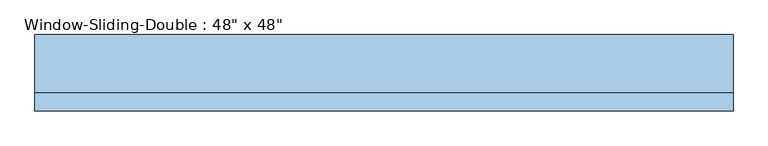
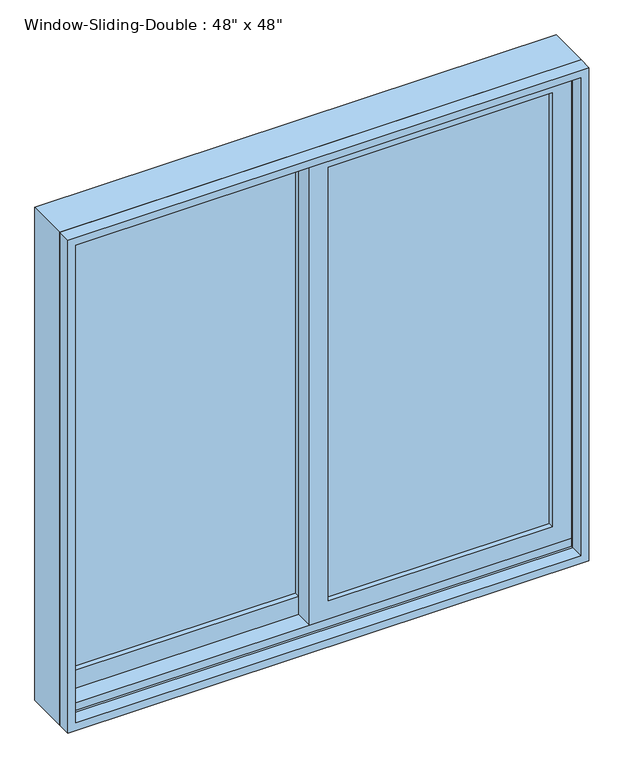
"""IFC4 building model written with IfcOpenShell, lengths in millimetres: window geometry."""

from ifc_helpers import new_model, si_unit, frame, origin, place, context, project, spatial, polyline, outline, extrude, faceted_brep, source, transform, mapped, element, save


def window_ba0d9a6f(model_context):
    return source(origin(), model_context, "Body", "SolidModel", [
        extrude(outline(polyline([(952.5, 590.55), (2114.55, 590.55), (2114.55, -22.225), (952.5, -22.225), (952.5, 590.55)]), holes=[polyline([(996.95, 22.225), (2070.1, 22.225), (2070.1, 546.1), (996.95, 546.1), (996.95, 22.225)])]), frame((0.0, -22.86, 0.0), z_axis=(0.0, 1.0, 0.0), x_axis=(0.0, 0.0, 1.0)), (0.0, 0.0, 1.0), 44.45),
        extrude(outline(polyline([(933.45, -590.55), (933.45, 22.225), (2114.55, 22.225), (2114.55, -590.55), (933.45, -590.55)]), holes=[polyline([(2070.1, -22.225), (996.95, -22.225), (996.95, -546.1), (2070.1, -546.1), (2070.1, -22.225)])]), frame((0.0, 21.59, 0.0), z_axis=(0.0, 1.0, 0.0), x_axis=(0.0, 0.0, 1.0)), (0.0, 0.0, 1.0), 44.45),
        extrude(outline(polyline([(-22.225, 53.34), (-22.225, 46.99), (-546.1, 46.99), (-546.1, 53.34), (-22.225, 53.34)])), frame((0.0, 0.0, 996.95), z_axis=(0.0, 0.0, 1.0), x_axis=(1.0, 0.0, 0.0)), (0.0, 0.0, 1.0), 1073.15),
        extrude(outline(polyline([(-22.225, 40.64), (-22.225, 34.29), (-546.1, 34.29), (-546.1, 40.64), (-22.225, 40.64)])), frame((0.0, 0.0, 996.95), z_axis=(0.0, 0.0, 1.0), x_axis=(1.0, 0.0, 0.0)), (0.0, 0.0, 1.0), 1073.15),
        extrude(outline(polyline([(546.1, 8.89), (546.1, 2.54), (22.225, 2.54), (22.225, 8.89), (546.1, 8.89)])), frame((0.0, 0.0, 996.95), z_axis=(0.0, 0.0, 1.0), x_axis=(1.0, 0.0, 0.0)), (0.0, 0.0, 1.0), 1073.15),
        extrude(outline(polyline([(546.1, -3.81), (546.1, -10.16), (22.225, -10.16), (22.225, -3.81), (546.1, -3.81)])), frame((0.0, 0.0, 996.95), z_axis=(0.0, 0.0, 1.0), x_axis=(1.0, 0.0, 0.0)), (0.0, 0.0, 1.0), 1073.15),
        extrude(outline(polyline([(2133.6, -609.6), (914.4, -609.6), (914.4, 609.6), (2133.6, 609.6), (2133.6, -609.6)]), holes=[polyline([(2114.55, 590.55), (933.45, 590.55), (933.45, -590.55), (2114.55, -590.55), (2114.55, 590.55)])]), frame((0.0, -60.96, 0.0), z_axis=(0.0, 1.0, 0.0), x_axis=(0.0, 0.0, 1.0)), (0.0, 0.0, 1.0), 31.75),
        faceted_brep([(-609.6, -29.21, 914.4), (-609.6, 72.39, 914.4), (609.6, 72.39, 914.4), (609.6, -29.21, 914.4), (-568.6778905, 72.39, 2092.6778905), (-568.6778905, 66.04, 2092.6778905), (-568.6778905, 66.04, 933.45), (-568.6778905, 72.39, 933.45), (568.6778905, 66.04, 2092.6778905), (568.6778905, 66.04, 933.45), (590.55, 66.04, 933.45), (590.55, 66.04, 2114.55), (-590.55, 66.04, 2114.55), (-590.55, 66.04, 933.45), (-590.55, -29.21, 2114.55), (-590.55, -29.21, 933.45), (-590.55, -22.86, 933.45), (-590.55, -22.86, 952.5), (-590.55, 21.59, 952.5), (-590.55, 21.59, 933.45), (609.6, -29.21, 2133.6), (-609.6, -29.21, 2133.6), (590.55, -29.21, 2114.55), (590.55, -29.21, 933.45), (-609.6, 72.39, 2133.6), (609.6, 72.39, 2133.6), (568.6778905, 72.39, 933.45), (568.6778905, 72.39, 2092.6778905), (590.55, 21.59, 933.45), (590.55, 21.59, 952.5), (590.55, -22.86, 952.5), (590.55, -22.86, 933.45)], [[[0, 1, 2, 3]], [[4, 5, 6, 7]], [[5, 8, 9, 10, 11, 12, 13, 6]], [[12, 14, 15, 16, 17, 18, 19, 13]], [[0, 3, 20, 21], [22, 23, 15, 14]], [[24, 1, 0, 21]], [[2, 1, 24, 25], [4, 7, 26, 27]], [[5, 4, 27, 8]], [[12, 11, 22, 14]], [[21, 20, 25, 24]], [[8, 27, 26, 9]], [[22, 11, 10, 28, 29, 30, 31, 23]], [[20, 3, 2, 25]], [[26, 7, 6, 13, 19, 28, 10, 9]], [[28, 19, 18, 29]], [[29, 18, 17, 30]], [[30, 17, 16, 31]], [[15, 23, 31, 16]]]),
    ])


if __name__ == "__main__":
    model = new_model("IFC4")
    model_context = context("Model", 3, world=origin())
    ifc_project = project(units=[si_unit("LENGTHUNIT", "METRE", prefix="MILLI")], contexts=[model_context])
    site = spatial("IfcSite", under=ifc_project)
    building = spatial("IfcBuilding", under=site)
    placement = place(None, origin())
    window_shape = window_ba0d9a6f(model_context)
    element("IfcWindow", 1, ObjectType="Window-Sliding-Double : 48\" x 48\"", at=placement, inside=building, context=model_context, shape_type="MappedRepresentation", body=[
        mapped(window_shape, transform((0.0, 0.0, 0.0), x_axis=(1.0, 0.0, 0.0), y_axis=(0.0, 1.0, 0.0), z_axis=(0.0, 0.0, 1.0))),
    ])
    save(model, "model.ifc")

# Revit data of these elements
# Type "Window-Sliding-Double : 48\" x 48\""
#   Type Mark = "22"
#   Fire Rating = "0.5h"
#   Assembly Code = "B2020100"
#   Analytic Construction = "Double glazing - domestic"
#   Window Inset [instance default] = 0' - 0"
#   Wall Thickness [instance default] = 0' - 6"
#   Visual Light Transmittance = 0.81
#   Thermal Resistance (R) = 1.8146 (h·ft²·°F)/BTU
#   Solar Heat Gain Coefficient = 0.76
#   Muntin Width = 1' - 8 5/8"
#   Muntin Height = 3' - 6 1/4"
#   Interior Wall Closure [instance default] = 0' - 2 3/4"
#   Heat Transfer Coefficient (U) = 0.5511 BTU/(h·ft²·°F)
#   Frame Extension [instance default] = 0' - 0 1/4"
#   Exterior Wall Closure [instance default] = 0' - 1 1/4"
#   Rough Width = 4' - 0 1/2"
#   Rough Height = 4' - 0 1/2"
#   Height = 4' - 0"
#   Extension Jamb [instance default] = 0' - 2 3/4"
#   Default Sill Height = 3' - 0"
#   Width = 4' - 0"
#   Interior Trim Visibility [instance default] = yes
#   Indicator Visibility [instance default] = yes
#   Exterior Trim Visibility [instance default] = yes
#   Muntin Visibility = yes
#   Extension Jamb Visibility [instance default] = yes
#   Muntin Pattern = Muntin Pattern_2x2 : Muntin Pattern_2x2
#   Interior Trim Material = Wood - Stained
#   Interior Trim = Trim-Window-Interior-Flat : Picture Frame
#   Interior Frame Material = Wood - Stained
#   Glass Panel Material = Glass
#   Exterior Trim Material = Clad - White
#   Exterior Trim = Trim-Window-Exterior-Flat : with Sill
#   Exterior Frame Material = Clad - White
#   Wall Closure = (empty or 0)
# Element 1 (IfcWindow, "Window-Sliding-Double : 48\" x 48\"")
#   Wall Thickness = 0' - 4 1/2"
#   Extension Jamb = 0' - 1 1/4"
#   Materials on its faces: "Wood - Stained", "Glass", "Clad - White"
# Materials
#   "Wood - Stained": class "Wood", colour RGB 224 178 126, transparency 0, Cost = 0
#   "Glass": class "Glass", colour RGB 0 128 192, transparency 0.75, Description = "Soda Lime Glass", Cost = 0
#   "Clad - White": class "Wood", colour RGB 242 242 238, transparency 0, Cost = 0
